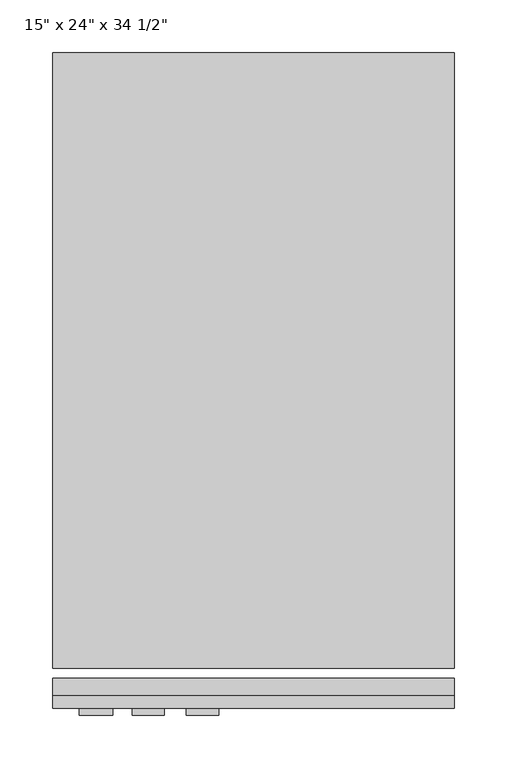
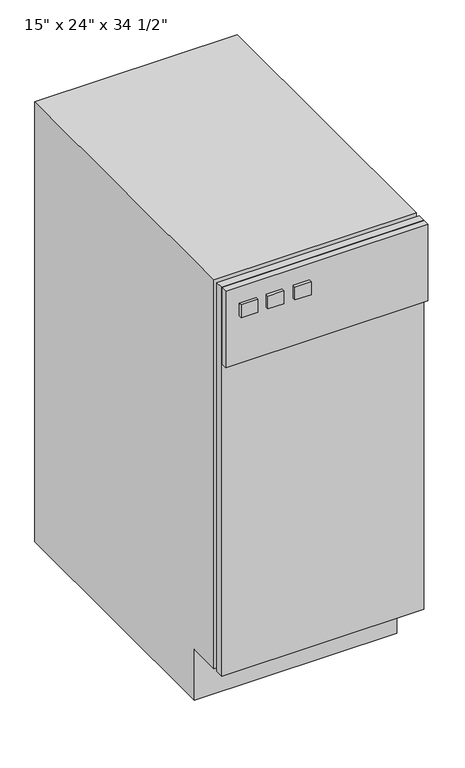
"""IFC4 building model written with IfcOpenShell, lengths in millimetres: proxy geometry."""

from ifc_helpers import new_model, si_unit, frame, origin, place, context, project, spatial, polyline, outline, extrude, source, transform, mapped, element, save


def proxy_db4bb64d(model_context):
    return source(origin(), model_context, "Body", "SweptSolid", [
        extrude(outline(polyline([(458.5174685, -38.3504352), (77.5174685, -38.3504352), (77.5174685, -22.4754352), (458.5174685, -22.4754352), (458.5174685, -38.3504352)])), frame((0.0, 0.0, 101.6), z_axis=(0.0, 0.0, 1.0), x_axis=(1.0, 0.0, 0.0)), (0.0, 0.0, 1.0), 774.7),
        extrude(outline(polyline([(458.5174685, -38.3504352), (458.5174685, -51.0504352), (77.5174685, -51.0504352), (77.5174685, -38.3504352), (458.5174685, -38.3504352)])), frame((0.0, 0.0, 723.9), z_axis=(0.0, 0.0, 1.0), x_axis=(1.0, 0.0, 0.0)), (0.0, 0.0, 1.0), 152.4),
        extrude(outline(polyline([(571.2495648, 0.0), (50.5495648, 0.0), (50.5495648, 101.6), (-12.9504352, 101.6), (-12.9504352, 876.3), (571.2495648, 876.3), (571.2495648, 0.0)])), frame((77.5174685, 0.0, 0.0), z_axis=(1.0, 0.0, 0.0), x_axis=(0.0, 1.0, 0.0)), (0.0, 0.0, 1.0), 381.0),
        extrude(outline(polyline([(134.6674685, -57.4004352), (102.9174685, -57.4004352), (102.9174685, -51.0504352), (134.6674685, -51.0504352), (134.6674685, -57.4004352)])), frame((0.0, 0.0, 818.6415009), z_axis=(0.0, 0.0, 1.0), x_axis=(1.0, 0.0, 0.0)), (0.0, 0.0, 1.0), 25.4),
        extrude(outline(polyline([(183.5847918, -57.4004352), (153.2389562, -57.4004352), (153.2389562, -51.0504352), (183.5847918, -51.0504352), (183.5847918, -57.4004352)])), frame((0.0, 0.0, 818.6415009), z_axis=(0.0, 0.0, 1.0), x_axis=(1.0, 0.0, 0.0)), (0.0, 0.0, 1.0), 25.4),
        extrude(outline(polyline([(234.869254, -57.4004352), (204.2199601, -57.4004352), (204.2199601, -51.0504352), (234.869254, -51.0504352), (234.869254, -57.4004352)])), frame((0.0, 0.0, 818.6415009), z_axis=(0.0, 0.0, 1.0), x_axis=(1.0, 0.0, 0.0)), (0.0, 0.0, 1.0), 25.4),
    ])


if __name__ == "__main__":
    model = new_model("IFC4")
    model_context = context("Model", 3, world=origin())
    ifc_project = project(units=[si_unit("LENGTHUNIT", "METRE", prefix="MILLI")], contexts=[model_context])
    site = spatial("IfcSite", under=ifc_project)
    building = spatial("IfcBuilding", under=site)
    placement = place(None, origin())
    proxy_shape = proxy_db4bb64d(model_context)
    element("IfcBuildingElementProxy", 1, Name="15\" x 24\" x 34 1/2\"", ObjectType="15\" x 24\" x 34 1/2\"", at=placement, inside=building, context=model_context, shape_type="MappedRepresentation", body=[
        mapped(proxy_shape, transform((0.0, 0.0, 0.0), x_axis=(1.0, 0.0, 0.0), y_axis=(0.0, 1.0, 0.0), z_axis=(0.0, 0.0, 1.0))),
    ])
    save(model, "model.ifc")

# Revit data of these elements
# Type "15\" x 24\" x 34 1/2\""
#   Label = "T"
#   Assembly Code = "E1090400"
#   Depth = 2' - 0"
#   Height = 2' - 10 1/2"
#   Width = 1' - 3"
#   Panel Face Material = Plastic, Opaque Black
#   Trach Compact. Material = Steel, Paint Finish, Ivory, Matte
#   Default Elevation = 0
# Element 1 (IfcBuildingElementProxy, "15\" x 24\" x 34 1/2\"")
#   Materials on its faces: "Steel, Paint Finish, Ivory, Matte", "Plastic, Opaque Black"
# Materials
#   "Plastic, Opaque Black": class "Plastic", colour RGB 0 0 0, transparency 0, Description = "Plastic, generic, opaque black", Cost = 0
#   "Steel, Paint Finish, Ivory, Matte": class "Metal", colour RGB 247 247 239, transparency 0, Description = "Steel, paint finish, ivory, matte", Cost = 0
